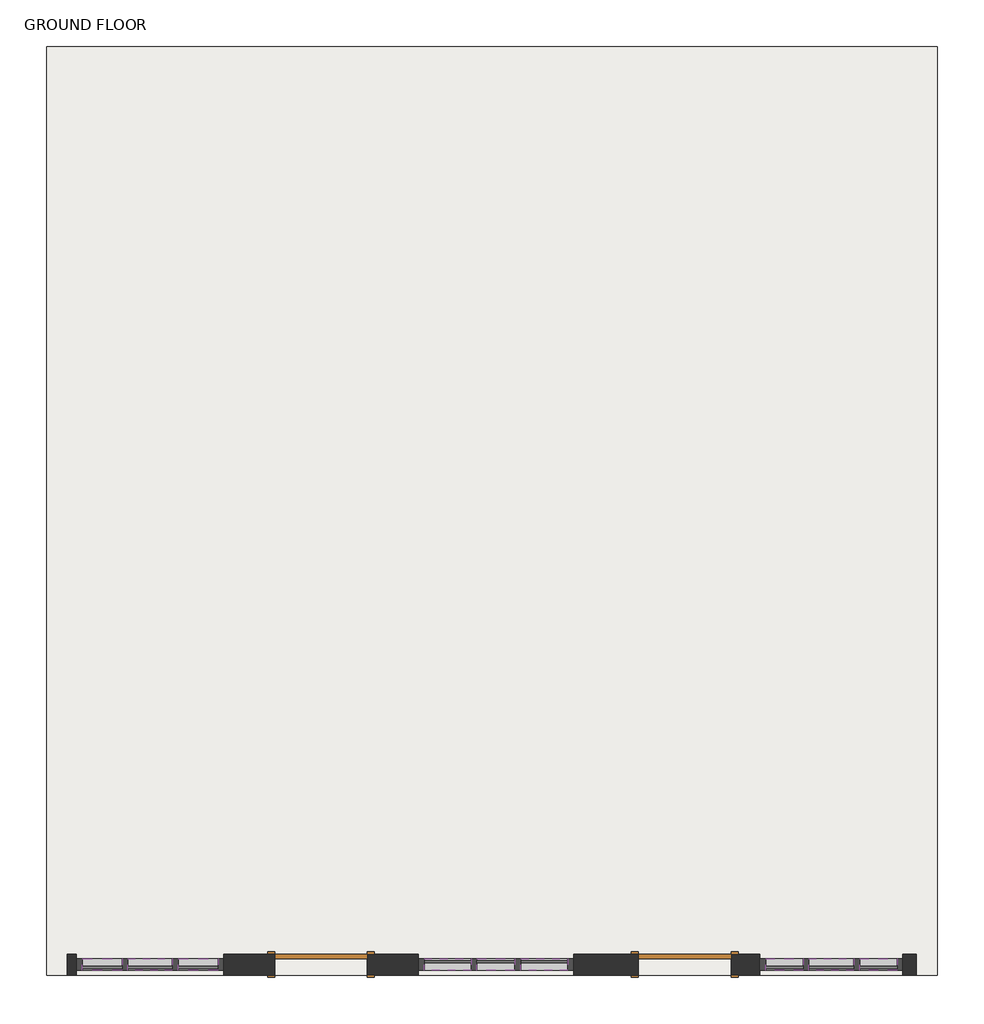
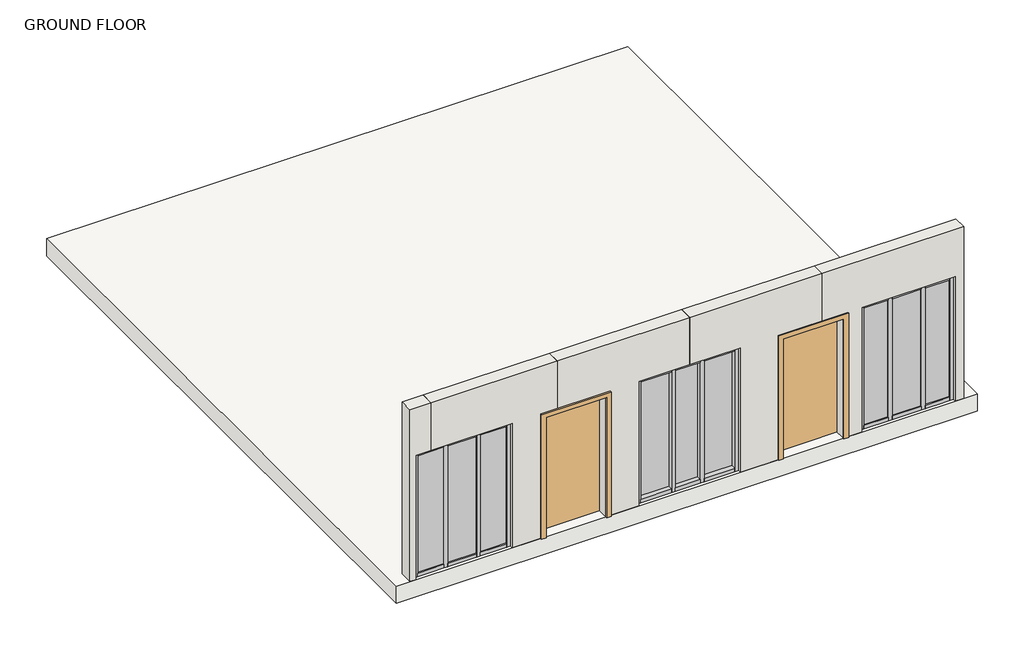
# One storey: 30 members, 9 plates, 5 walls, 2 doors, 1 slab.
"""IFC4 building model written with IfcOpenShell, lengths in millimetres."""

from ifc_helpers import new_model, si_unit, frame, origin, place, context, project, spatial, polyline, outline, extrude, transform, mapped, element, save
from components import single_flush_md_00354a0c, single_flush_md_8244dad1, member_76111e69, member_1182c56c, member_0b7646a3, member_5a7758d4, member_6fb4a552, member_d55fe2b3, member_dc106669, member_285d49a4, system_panel_glazed_e322ed92, system_panel_glazed_b4366bb5, system_panel_glazed_1118b51c, system_panel_glazed_5e4042f1, system_panel_glazed_8c9d9dbc, system_panel_glazed_b4762422

model = new_model("IFC4")

# Units and contexts
model_context = context("Model", 3, world=origin())
ifc_project = project(units=[si_unit("LENGTHUNIT", "METRE", prefix="MILLI")], contexts=[model_context])

# Site, building, storey
site = spatial("IfcSite", under=ifc_project)
building = spatial("IfcBuilding", under=site)
storey = spatial("IfcBuildingStorey", under=building, Name="GROUND FLOOR", Elevation=0.0)

# Doors
placement = place(None, origin())
single_flush_md_shape = single_flush_md_00354a0c(model_context)
element("IfcDoor", 1, ObjectType="Single-Flush : md", at=placement, inside=storey, context=model_context, shape_type="MappedRepresentation", body=[
    mapped(single_flush_md_shape, transform((-3316.8029969, -1153.2217235, 0.0), x_axis=(1.0, 0.0, 0.0), y_axis=(0.0, 1.0, 0.0), z_axis=(0.0, 0.0, 1.0))),
])
single_flush_md_2_shape = single_flush_md_8244dad1(model_context)
element("IfcDoor", 2, ObjectType="Single-Flush : md", at=placement, inside=storey, context=model_context, shape_type="MappedRepresentation", body=[
    mapped(single_flush_md_2_shape, transform((668.544858, -1153.2217235, 0.0), x_axis=(-1.0, 0.0, 0.0), y_axis=(0.0, -1.0, 0.0), z_axis=(0.0, 0.0, 1.0))),
])

# Members
member_shape = member_76111e69(model_context)
element("IfcMember", 3, ObjectType="Rectangular Mullion : 2.5\" x 5\" rectangular", at=placement, inside=storey, context=model_context, shape_type="MappedRepresentation", body=[
    mapped(member_shape, transform((-4378.9230786, -1153.2217235, 0.0), x_axis=(1.0, 0.0, 0.0), y_axis=(0.0, -1.0, 0.0), z_axis=(0.0, 0.0, -1.0))),
])
element("IfcMember", 4, ObjectType="Rectangular Mullion : 2.5\" x 5\" rectangular", at=placement, inside=storey, context=model_context, shape_type="MappedRepresentation", body=[
    mapped(member_shape, transform((3057.8150219, -1153.2217235, 0.0), x_axis=(1.0, 0.0, 0.0), y_axis=(0.0, -1.0, 0.0), z_axis=(0.0, 0.0, -1.0))),
])
element("IfcMember", 5, ObjectType="Rectangular Mullion : 2.5\" x 5\" rectangular", at=placement, inside=storey, context=model_context, shape_type="MappedRepresentation", body=[
    mapped(member_shape, transform((-5996.2451909, -1153.2217235, 2209.8), x_axis=(-1.0, 0.0, 0.0), y_axis=(0.0, -1.0, 0.0), z_axis=(0.0, 0.0, 1.0))),
])
element("IfcMember", 6, ObjectType="Rectangular Mullion : 2.5\" x 5\" rectangular", at=placement, inside=storey, context=model_context, shape_type="MappedRepresentation", body=[
    mapped(member_shape, transform((1488.4769214, -1153.2217235, 2209.8), x_axis=(-1.0, 0.0, 0.0), y_axis=(0.0, -1.0, 0.0), z_axis=(0.0, 0.0, 1.0))),
])
element("IfcMember", 7, ObjectType="Rectangular Mullion : 2.5\" x 5\" rectangular", at=placement, inside=storey, context=model_context, shape_type="MappedRepresentation", body=[
    mapped(member_shape, transform((-550.655142, -1153.2217235, 0.0), x_axis=(1.0, 0.0, 0.0), y_axis=(0.0, -1.0, 0.0), z_axis=(0.0, 0.0, -1.0))),
])
element("IfcMember", 8, ObjectType="Rectangular Mullion : 2.5\" x 5\" rectangular", at=placement, inside=storey, context=model_context, shape_type="MappedRepresentation", body=[
    mapped(member_shape, transform((-2250.0029969, -1153.2217235, 2209.8), x_axis=(-1.0, 0.0, 0.0), y_axis=(0.0, -1.0, 0.0), z_axis=(0.0, 0.0, 1.0))),
])
member_2_shape = member_1182c56c(model_context)
element("IfcMember", 9, ObjectType="Rectangular Mullion : 2.5\" x 5\" rectangular", at=placement, inside=storey, context=model_context, shape_type="MappedRepresentation", body=[
    mapped(member_2_shape, transform((-1640.4029969, -1153.2217235, 0.0), x_axis=(1.0, 0.0, 0.0), y_axis=(0.0, -1.0, 0.0), z_axis=(0.0, 0.0, -1.0))),
])
element("IfcMember", 10, ObjectType="Rectangular Mullion : 2.5\" x 5\" rectangular", at=placement, inside=storey, context=model_context, shape_type="MappedRepresentation", body=[
    mapped(member_2_shape, transform((-1160.255142, -1153.2217235, 0.0), x_axis=(1.0, 0.0, 0.0), y_axis=(0.0, -1.0, 0.0), z_axis=(0.0, 0.0, -1.0))),
])
member_3_shape = member_0b7646a3(model_context)
element("IfcMember", 11, ObjectType="Rectangular Mullion : 2.5\" x 5\" rectangular", at=placement, inside=storey, context=model_context, shape_type="MappedRepresentation", body=[
    mapped(member_3_shape, transform((-2186.5029969, -1153.2217235, 0.0), x_axis=(0.0, 0.0, -1.0), y_axis=(0.0, -1.0, 0.0), z_axis=(-1.0, 0.0, 0.0))),
])
element("IfcMember", 12, ObjectType="Rectangular Mullion : 2.5\" x 5\" rectangular", at=placement, inside=storey, context=model_context, shape_type="MappedRepresentation", body=[
    mapped(member_3_shape, transform((-1128.505142, -1153.2217235, 0.0), x_axis=(0.0, 0.0, -1.0), y_axis=(0.0, -1.0, 0.0), z_axis=(-1.0, 0.0, 0.0))),
])
element("IfcMember", 13, ObjectType="Rectangular Mullion : 2.5\" x 5\" rectangular", at=placement, inside=storey, context=model_context, shape_type="MappedRepresentation", body=[
    mapped(member_3_shape, transform((-614.155142, -1153.2217235, 2209.8), x_axis=(0.0, 0.0, 1.0), y_axis=(0.0, -1.0, 0.0), z_axis=(1.0, 0.0, 0.0))),
])
element("IfcMember", 14, ObjectType="Rectangular Mullion : 2.5\" x 5\" rectangular", at=placement, inside=storey, context=model_context, shape_type="MappedRepresentation", body=[
    mapped(member_3_shape, transform((-1672.1529969, -1153.2217235, 2209.8), x_axis=(0.0, 0.0, 1.0), y_axis=(0.0, -1.0, 0.0), z_axis=(1.0, 0.0, 0.0))),
])
member_4_shape = member_5a7758d4(model_context)
element("IfcMember", 15, ObjectType="Rectangular Mullion : 2.5\" x 5\" rectangular", at=placement, inside=storey, context=model_context, shape_type="MappedRepresentation", body=[
    mapped(member_4_shape, transform((-1608.6529969, -1153.2217235, 0.0), x_axis=(0.0, 0.0, -1.0), y_axis=(0.0, -1.0, 0.0), z_axis=(-1.0, 0.0, 0.0))),
])
element("IfcMember", 16, ObjectType="Rectangular Mullion : 2.5\" x 5\" rectangular", at=placement, inside=storey, context=model_context, shape_type="MappedRepresentation", body=[
    mapped(member_4_shape, transform((-1192.005142, -1153.2217235, 2209.8), x_axis=(0.0, 0.0, 1.0), y_axis=(0.0, -1.0, 0.0), z_axis=(1.0, 0.0, 0.0))),
])
element("IfcMember", 17, ObjectType="Rectangular Mullion : 2.5\" x 5\" rectangular", at=placement, inside=storey, context=model_context, shape_type="MappedRepresentation", body=[
    mapped(member_2_shape, transform((-5462.8451909, -1153.2217235, 0.0), x_axis=(1.0, 0.0, 0.0), y_axis=(0.0, -1.0, 0.0), z_axis=(0.0, 0.0, -1.0))),
])
element("IfcMember", 18, ObjectType="Rectangular Mullion : 2.5\" x 5\" rectangular", at=placement, inside=storey, context=model_context, shape_type="MappedRepresentation", body=[
    mapped(member_2_shape, transform((-4912.3230786, -1153.2217235, 0.0), x_axis=(1.0, 0.0, 0.0), y_axis=(0.0, -1.0, 0.0), z_axis=(0.0, 0.0, -1.0))),
])
element("IfcMember", 19, ObjectType="Rectangular Mullion : 2.5\" x 5\" rectangular", at=placement, inside=storey, context=model_context, shape_type="MappedRepresentation", body=[
    mapped(member_2_shape, transform((1996.4769214, -1153.2217235, 0.0), x_axis=(1.0, 0.0, 0.0), y_axis=(0.0, -1.0, 0.0), z_axis=(0.0, 0.0, -1.0))),
])
element("IfcMember", 20, ObjectType="Rectangular Mullion : 2.5\" x 5\" rectangular", at=placement, inside=storey, context=model_context, shape_type="MappedRepresentation", body=[
    mapped(member_2_shape, transform((2549.8150219, -1153.2217235, 0.0), x_axis=(1.0, 0.0, 0.0), y_axis=(0.0, -1.0, 0.0), z_axis=(0.0, 0.0, -1.0))),
])
member_5_shape = member_6fb4a552(model_context)
element("IfcMember", 21, ObjectType="Rectangular Mullion : 2.5\" x 5\" rectangular", at=placement, inside=storey, context=model_context, shape_type="MappedRepresentation", body=[
    mapped(member_5_shape, transform((-5932.7451909, -1153.2217235, 0.0), x_axis=(0.0, 0.0, -1.0), y_axis=(0.0, -1.0, 0.0), z_axis=(-1.0, 0.0, 0.0))),
])
element("IfcMember", 22, ObjectType="Rectangular Mullion : 2.5\" x 5\" rectangular", at=placement, inside=storey, context=model_context, shape_type="MappedRepresentation", body=[
    mapped(member_5_shape, transform((-4880.5730786, -1153.2217235, 0.0), x_axis=(0.0, 0.0, -1.0), y_axis=(0.0, -1.0, 0.0), z_axis=(-1.0, 0.0, 0.0))),
])
element("IfcMember", 23, ObjectType="Rectangular Mullion : 2.5\" x 5\" rectangular", at=placement, inside=storey, context=model_context, shape_type="MappedRepresentation", body=[
    mapped(member_5_shape, transform((-4442.4230786, -1153.2217235, 2209.8), x_axis=(0.0, 0.0, 1.0), y_axis=(0.0, -1.0, 0.0), z_axis=(1.0, 0.0, 0.0))),
])
element("IfcMember", 24, ObjectType="Rectangular Mullion : 2.5\" x 5\" rectangular", at=placement, inside=storey, context=model_context, shape_type="MappedRepresentation", body=[
    mapped(member_5_shape, transform((-5494.5951909, -1153.2217235, 2209.8), x_axis=(0.0, 0.0, 1.0), y_axis=(0.0, -1.0, 0.0), z_axis=(1.0, 0.0, 0.0))),
])
member_6_shape = member_d55fe2b3(model_context)
element("IfcMember", 25, ObjectType="Rectangular Mullion : 2.5\" x 5\" rectangular", at=placement, inside=storey, context=model_context, shape_type="MappedRepresentation", body=[
    mapped(member_6_shape, transform((-5431.0951909, -1153.2217235, 0.0), x_axis=(0.0, 0.0, -1.0), y_axis=(0.0, -1.0, 0.0), z_axis=(-1.0, 0.0, 0.0))),
])
element("IfcMember", 26, ObjectType="Rectangular Mullion : 2.5\" x 5\" rectangular", at=placement, inside=storey, context=model_context, shape_type="MappedRepresentation", body=[
    mapped(member_6_shape, transform((-4944.0730786, -1153.2217235, 2209.8), x_axis=(0.0, 0.0, 1.0), y_axis=(0.0, -1.0, 0.0), z_axis=(1.0, 0.0, 0.0))),
])
member_7_shape = member_dc106669(model_context)
element("IfcMember", 27, ObjectType="Rectangular Mullion : 2.5\" x 5\" rectangular", at=placement, inside=storey, context=model_context, shape_type="MappedRepresentation", body=[
    mapped(member_7_shape, transform((1551.9769214, -1153.2217235, 0.0), x_axis=(0.0, 0.0, -1.0), y_axis=(0.0, -1.0, 0.0), z_axis=(-1.0, 0.0, 0.0))),
])
element("IfcMember", 28, ObjectType="Rectangular Mullion : 2.5\" x 5\" rectangular", at=placement, inside=storey, context=model_context, shape_type="MappedRepresentation", body=[
    mapped(member_7_shape, transform((2581.5650219, -1153.2217235, 0.0), x_axis=(0.0, 0.0, -1.0), y_axis=(0.0, -1.0, 0.0), z_axis=(-1.0, 0.0, 0.0))),
])
element("IfcMember", 29, ObjectType="Rectangular Mullion : 2.5\" x 5\" rectangular", at=placement, inside=storey, context=model_context, shape_type="MappedRepresentation", body=[
    mapped(member_7_shape, transform((2994.3150219, -1153.2217235, 2209.8), x_axis=(0.0, 0.0, 1.0), y_axis=(0.0, -1.0, 0.0), z_axis=(1.0, 0.0, 0.0))),
])
element("IfcMember", 30, ObjectType="Rectangular Mullion : 2.5\" x 5\" rectangular", at=placement, inside=storey, context=model_context, shape_type="MappedRepresentation", body=[
    mapped(member_7_shape, transform((1964.7269214, -1153.2217235, 2209.8), x_axis=(0.0, 0.0, 1.0), y_axis=(0.0, -1.0, 0.0), z_axis=(1.0, 0.0, 0.0))),
])
member_8_shape = member_285d49a4(model_context)
element("IfcMember", 31, ObjectType="Rectangular Mullion : 2.5\" x 5\" rectangular", at=placement, inside=storey, context=model_context, shape_type="MappedRepresentation", body=[
    mapped(member_8_shape, transform((2028.2269214, -1153.2217235, 0.0), x_axis=(0.0, 0.0, -1.0), y_axis=(0.0, -1.0, 0.0), z_axis=(-1.0, 0.0, 0.0))),
])
element("IfcMember", 32, ObjectType="Rectangular Mullion : 2.5\" x 5\" rectangular", at=placement, inside=storey, context=model_context, shape_type="MappedRepresentation", body=[
    mapped(member_8_shape, transform((2518.0650219, -1153.2217235, 2209.8), x_axis=(0.0, 0.0, 1.0), y_axis=(0.0, -1.0, 0.0), z_axis=(1.0, 0.0, 0.0))),
])

# Plates
system_panel_glazed_shape = system_panel_glazed_e322ed92(model_context)
element("IfcPlate", 33, ObjectType="System Panel : Glazed", at=placement, inside=storey, context=model_context, shape_type="MappedRepresentation", body=[
    mapped(system_panel_glazed_shape, transform((-1929.3279969, -1153.2217235, 63.5), x_axis=(1.0, 0.0, 0.0), y_axis=(0.0, 1.0, 0.0), z_axis=(0.0, 0.0, 1.0))),
])
element("IfcPlate", 34, ObjectType="System Panel : Glazed", at=placement, inside=storey, context=model_context, shape_type="MappedRepresentation", body=[
    mapped(system_panel_glazed_shape, transform((-871.330142, -1153.2217235, 63.5), x_axis=(1.0, 0.0, 0.0), y_axis=(0.0, 1.0, 0.0), z_axis=(0.0, 0.0, 1.0))),
])
system_panel_glazed_2_shape = system_panel_glazed_b4366bb5(model_context)
element("IfcPlate", 35, ObjectType="System Panel : Glazed", at=placement, inside=storey, context=model_context, shape_type="MappedRepresentation", body=[
    mapped(system_panel_glazed_2_shape, transform((-1400.3290695, -1153.2217235, 63.5), x_axis=(1.0, 0.0, 0.0), y_axis=(0.0, 1.0, 0.0), z_axis=(0.0, 0.0, 1.0))),
])
system_panel_glazed_3_shape = system_panel_glazed_1118b51c(model_context)
element("IfcPlate", 36, ObjectType="System Panel : Glazed", at=placement, inside=storey, context=model_context, shape_type="MappedRepresentation", body=[
    mapped(system_panel_glazed_3_shape, transform((-5713.6701909, -1153.2217235, 63.5), x_axis=(1.0, 0.0, 0.0), y_axis=(0.0, 1.0, 0.0), z_axis=(0.0, 0.0, 1.0))),
])
element("IfcPlate", 37, ObjectType="System Panel : Glazed", at=placement, inside=storey, context=model_context, shape_type="MappedRepresentation", body=[
    mapped(system_panel_glazed_3_shape, transform((-4661.4980786, -1153.2217235, 63.5), x_axis=(1.0, 0.0, 0.0), y_axis=(0.0, 1.0, 0.0), z_axis=(0.0, 0.0, 1.0))),
])
system_panel_glazed_4_shape = system_panel_glazed_5e4042f1(model_context)
element("IfcPlate", 38, ObjectType="System Panel : Glazed", at=placement, inside=storey, context=model_context, shape_type="MappedRepresentation", body=[
    mapped(system_panel_glazed_4_shape, transform((-5187.5841347, -1153.2217235, 63.5), x_axis=(1.0, 0.0, 0.0), y_axis=(0.0, 1.0, 0.0), z_axis=(0.0, 0.0, 1.0))),
])
system_panel_glazed_5_shape = system_panel_glazed_8c9d9dbc(model_context)
element("IfcPlate", 39, ObjectType="System Panel : Glazed", at=placement, inside=storey, context=model_context, shape_type="MappedRepresentation", body=[
    mapped(system_panel_glazed_5_shape, transform((1758.3519214, -1153.2217235, 63.5), x_axis=(1.0, 0.0, 0.0), y_axis=(0.0, 1.0, 0.0), z_axis=(0.0, 0.0, 1.0))),
])
element("IfcPlate", 40, ObjectType="System Panel : Glazed", at=placement, inside=storey, context=model_context, shape_type="MappedRepresentation", body=[
    mapped(system_panel_glazed_5_shape, transform((2787.9400219, -1153.2217235, 63.5), x_axis=(1.0, 0.0, 0.0), y_axis=(0.0, 1.0, 0.0), z_axis=(0.0, 0.0, 1.0))),
])
system_panel_glazed_6_shape = system_panel_glazed_b4762422(model_context)
element("IfcPlate", 41, ObjectType="System Panel : Glazed", at=placement, inside=storey, context=model_context, shape_type="MappedRepresentation", body=[
    mapped(system_panel_glazed_6_shape, transform((2273.1459717, -1153.2217235, 63.5), x_axis=(1.0, 0.0, 0.0), y_axis=(0.0, 1.0, 0.0), z_axis=(0.0, 0.0, 1.0))),
])

# Slab
element("IfcSlab", 42, ObjectType="Generic - 12\"", at=placement, inside=storey, context=model_context, shape_type="SweptSolid", body=[
    extrude(outline(polyline([(3431.5769214, -1267.5217235), (-6322.0230786, -1267.5217235), (-6322.0230786, 8902.3535822), (3431.5769214, 8902.3535822), (3431.5769214, -1267.5217235)])), frame((0.0, 0.0, -304.8), z_axis=(0.0, 0.0, 1.0), x_axis=(1.0, 0.0, 0.0)), (0.0, 0.0, 1.0), 304.8),
])

# Walls
element("IfcWall", 43, ObjectType="9\"", at=placement, inside=storey, context=model_context, shape_type="SweptSolid", body=[
    extrude(outline(polyline([(3048.0, -5742.2451909), (3048.0, -6093.4230786), (0.0, -6093.4230786), (0.0, -5996.2451909), (2209.8, -5996.2451909), (2209.8, -5742.2451909), (3048.0, -5742.2451909)])), frame((0.0, -1267.5217235, 0.0), z_axis=(0.0, 1.0, 0.0), x_axis=(0.0, 0.0, 1.0)), (0.0, 0.0, 1.0), 228.6),
])
element("IfcWall", 44, ObjectType="9\"", at=placement, inside=storey, context=model_context, shape_type="SweptSolid", body=[
    extrude(outline(polyline([(3048.0, -3621.6029969), (3048.0, -5742.2451909), (2209.8, -5742.2451909), (2209.8, -4378.9230786), (0.0, -4378.9230786), (0.0, -3824.8029969), (2133.6, -3824.8029969), (2133.6, -3621.6029969), (3048.0, -3621.6029969)])), frame((0.0, -1267.5217235, 0.0), z_axis=(0.0, 1.0, 0.0), x_axis=(0.0, 0.0, 1.0)), (0.0, 0.0, 1.0), 228.6),
])
element("IfcWall", 45, ObjectType="9\"", at=placement, inside=storey, context=model_context, shape_type="SweptSolid", body=[
    extrude(outline(polyline([(3048.0, 3202.9769214), (3048.0, 820.944858), (2133.6, 820.944858), (2133.6, 1176.544858), (0.0, 1176.544858), (0.0, 1488.4769214), (2209.8, 1488.4769214), (2209.8, 3057.8150219), (0.0, 3057.8150219), (0.0, 3202.9769214), (3048.0, 3202.9769214)])), frame((0.0, -1267.5217235, 0.0), z_axis=(0.0, 1.0, 0.0), x_axis=(0.0, 0.0, 1.0)), (0.0, 0.0, 1.0), 228.6),
])
element("IfcWall", 46, ObjectType="9\"", at=placement, inside=storey, context=model_context, shape_type="SweptSolid", body=[
    extrude(outline(polyline([(3048.0, -1400.3290695), (3048.0, -3621.6029969), (2133.6, -3621.6029969), (2133.6, -2808.8029969), (0.0, -2808.8029969), (0.0, -2250.0029969), (2209.8, -2250.0029969), (2209.8, -1400.3290695), (3048.0, -1400.3290695)])), frame((0.0, -1267.5217235, 0.0), z_axis=(0.0, 1.0, 0.0), x_axis=(0.0, 0.0, 1.0)), (0.0, 0.0, 1.0), 228.6),
])
element("IfcWall", 47, ObjectType="9\"", at=placement, inside=storey, context=model_context, shape_type="SweptSolid", body=[
    extrude(outline(polyline([(3048.0, 820.944858), (3048.0, -1400.3290695), (2209.8, -1400.3290695), (2209.8, -550.655142), (0.0, -550.655142), (0.0, 160.544858), (2133.6, 160.544858), (2133.6, 820.944858), (3048.0, 820.944858)])), frame((0.0, -1267.5217235, 0.0), z_axis=(0.0, 1.0, 0.0), x_axis=(0.0, 0.0, 1.0)), (0.0, 0.0, 1.0), 228.6),
])

save(model, "model.ifc")

# Revit data of these elements
# Type "Single-Flush : md"
#   Type Mark = "8"
#   Construction Type Id = "MDOOR"
#   Assembly Code = "C1020"
#   Analytic Construction = "Metal"
#   Thickness = 0' - 2"
#   Heat Transfer Coefficient (U) = 0.651978 BTU/(h·ft²·°F)
#   Height = 7' - 0"
#   Trim Projection Ext = 0' - 1"
#   Trim Projection Int = 0' - 1"
#   Trim Width = 0' - 3"
#   Width = 3' - 4"
#   Define Thermal Properties by = 1
#   Door Material = Door - Panel
#   Frame Material = Door - Frame
#   Visual Light Transmittance = 0
#   Solar Heat Gain Coefficient = 0
#   Function = (empty or 0)
#   Wall Closure = (empty or 0)
# Type "Rectangular Mullion : 2.5\" x 5\" rectangular"
#   built-in parameter 1007304 = 0.416667 (stored number, unit not read)
#   built-in parameter 1007301 = 0.104167 (stored number, unit not read)
#   built-in parameter 1007300 = 0.104167 (stored number, unit not read)
# Type "System Panel : Glazed"
#   Construction Type Id = "GSP4R"
#   Analytic Construction = "1/8 in Pilkington single glazing"
#   Visual Light Transmittance = 0.9
#   Solar Heat Gain Coefficient = 0.86
#   Heat Transfer Coefficient (U) = 1.18115 BTU/(h·ft²·°F)
#   Define Thermal Properties by = 1
# Type "Generic - 12\""
#   Assembly Code = "B1010"
#   Function = 0
#   Layers, outside or top first: 1' - 0" no material (function 1)
# Type "9\""
#   Assembly Code = "B2010"
#   Layers, outside or top first: 0' - 9" no material (function 1)
# Elements 1, 2 (IfcDoor, "Single-Flush : md")
#   Phase Created = New Construction
#   Materials on its faces: "Door - Frame", "Door - Panel"
# Elements 3, 4, 5, 6, 7, 8, 9, 10, 11, 12, 13, 14, 15, 16, 17, 18, 19, 20, 21, 22, 23, 24, 25, 26, 27, 28, 29, 30, 31, 32 (IfcMember, "Rectangular Mullion : 2.5\" x 5\" rectangular")
#   Phase Created = New Construction
#   Materials on its faces: "Aluminum"
# Elements 33, 34, 35, 36, 37, 38, 39, 40, 41 (IfcPlate, "System Panel : Glazed")
#   Phase Created = New Construction
#   Materials on its faces: "Glass"
# Element 42 (IfcSlab, "Generic - 12\"")
#   Height Offset From Level = 0' - 0"
#   Phase Created = New Construction
#   Materials on its faces: "Default Floor"
# Elements 43, 44, 45, 46, 47 (IfcWall, "9\"")
#   Top Offset = 0' - 0"
#   Base Offset = 0' - 0"
#   Unconnected Height = 10' - 0"
#   wall height = 10' - 0"
#   Phase Created = New Construction
#   Base Constraint = GROUND FLOOR
#   Materials on its faces: "Default Wall", "1 wall"
# Materials
#   "Door - Panel": class "Wood", colour RGB 210 159 95, transparency 0, Cost = 0
#   "Door - Frame": colour RGB 118 70 51, transparency 0, Cost = 0
#   "Aluminum": class "Metal", colour RGB 247 247 247, transparency 0, Description = "Aluminum 6061", Cost = 0
#   "Glass": class "Glass", colour RGB 0 128 192, transparency 0.75, Description = "Soda Lime Glass", Cost = 0
#   "Default Floor": colour RGB 128 128 128, transparency 0, Cost = 0
#   "Default Wall": colour RGB 128 128 128, transparency 0, Cost = 0
#   "1 wall": class "Generic", colour RGB 244 245 241, transparency 0, Cost = 0
